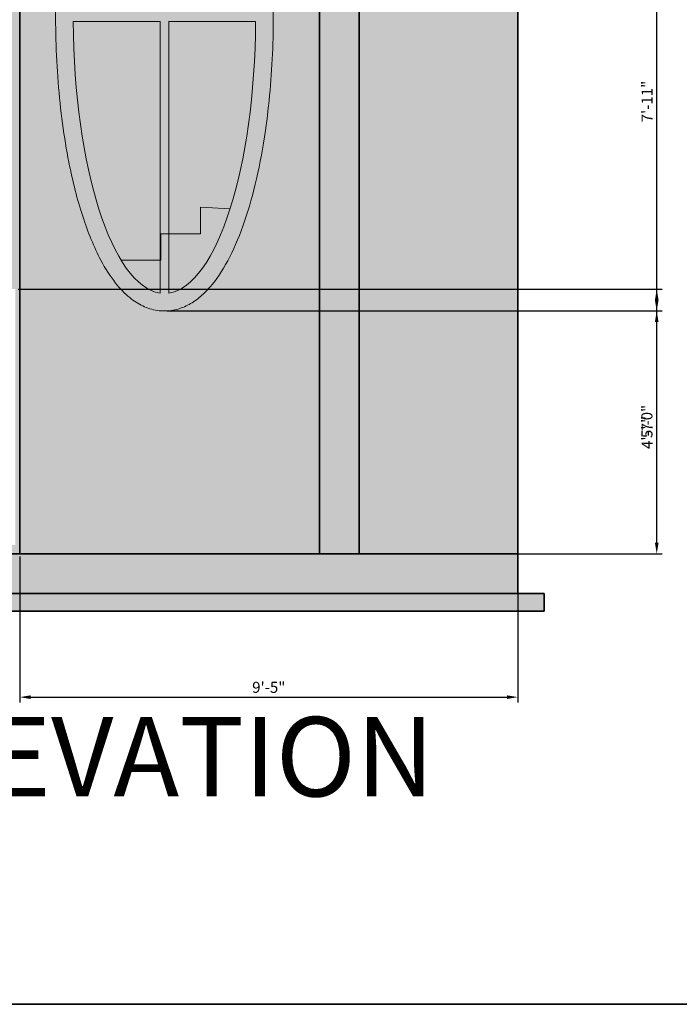
# Model space of a CAD drawing. Units: inches. Extents: x 2150 to 10686, y 1035 to 5077.
# Tile 6 of 12: x 6368 to 6517, y 4201 to 4425. Entities that reach past the tile are written whole.
import ezdxf

# ---------------------------------------------------------------- set-up
doc = ezdxf.new("R2010")
doc.units = ezdxf.units.IN
for name, color, linetype, lineweight in [('A-ANNO-DIMS', 2, 'Continuous', 18), ('A-ANNO-TITL', 3, 'Continuous', 35), ('A-ANNO-TTLB', 7, 'Continuous', 35), ('A-ELEV', 7, 'Continuous', 35), ('A-ELEV-BASE-PATT', 251, 'Continuous', 13), ('A-ELEV-GLAZ', 7, 'Continuous', 18), ('A-ELEV-METL-PATT', 252, 'Continuous', 13), ('A-ELEV-STRS', 7, 'Continuous', 18)]:
    doc.layers.add(name, color=color, linetype=linetype, lineweight=lineweight)
for name, color, linetype, lineweight, true_color in [('A-ELEV-CONC-PATT', 253, 'Continuous', 13, 0xb2a88f), ('A-ELEV-GLAZ-PATT', 141, 'Continuous', 13, 0xadddf7), ('A-ELEV-PATT', 253, 'Continuous', 13, 0xa5adc8), ('A-ELEV-TRIM-PATT', 85, 'Continuous', 13, 0x58ba48)]:
    doc.layers.add(name, color=color, linetype=linetype, lineweight=lineweight, true_color=true_color)
doc.styles.get("Standard").update_dxf_attribs({"font": 'arial.ttf'})
doc.dimstyles.new('ISO-25', dxfattribs={"dimtxt": 2.5, "dimasz": 2.5, "dimexe": 1.25, "dimexo": 0.625, "dimtad": 1, "dimdec": 0, "dimlunit": 3, "dimtxsty": 'Standard', "dimcen": 2.5, "dimadec": 0, "dimazin": 0, "dimtfac": 1, "dimtdec": 0, "dimtmove": 0, "dimatfit": 3, "dimfxl": 1, "dimarcsym": 0})

# ---------------------------------------------------------------- blocks, each defined once
blk = doc.blocks.new('*D130')
at = {"layer": 'A-ANNO-DIMS', "color": 0, "lineweight": -2, "transparency": 16777216}
for p, q in [((6401.069858000004, 4358.524472000001), (6513.357663000007, 4358.524472000001)), ((6512.107663000008, 4305.984460000001), (6512.107663000008, 4356.024472000002)), ((6481.232663000003, 4303.484460000001), (6513.357663000007, 4303.484460000001))]:
    blk.add_line(p, q, dxfattribs=at)
at = {"layer": 'A-ANNO-DIMS', "color": 0, "transparency": 16777216}
for points in [[(6511.69099633334, 4356.024472000002), (6512.524329666674, 4356.024472000002), (6512.107663000008, 4358.524472000001)], [(6511.69099633334, 4305.984460000001), (6512.524329666674, 4305.984460000001), (6512.107663000008, 4303.484460000001)]]:
    blk.add_solid(points, dxfattribs=at)
at = {"layer": 'Defpoints', "color": 0, "transparency": 16777216}
for p in [(6400.444858000003, 4358.524472000001), (6512.107663000008, 4358.524472000001), (6480.607663000004, 4303.484460000001)]:
    blk.add_point(p, dxfattribs=at)
at = {"layer": 'A-ANNO-DIMS', "color": 0, "transparency": 16777216, "insert": (6510.232663000007, 4331.004465999998), "char_height": 2.5, "attachment_point": 5, "rotation": 90}
blk.add_mtext('4\'-7"', dxfattribs=at)
blk = doc.blocks.new('*D131')
at = {"layer": 'A-ANNO-DIMS', "color": 0, "lineweight": -2, "transparency": 16777216}
for p, q in [((6493.232663000004, 4453.484460000001), (6513.357663000007, 4453.484460000001)), ((6512.107663000008, 4361.024472000002), (6512.107663000008, 4450.984460000001)), ((6401.069858000004, 4358.524472000001), (6513.357663000007, 4358.524472000001))]:
    blk.add_line(p, q, dxfattribs=at)
at = {"layer": 'A-ANNO-DIMS', "color": 0, "transparency": 16777216}
for points in [[(6511.69099633334, 4450.984460000001), (6512.524329666674, 4450.984460000001), (6512.107663000008, 4453.484460000001)], [(6511.69099633334, 4361.024472000002), (6512.524329666674, 4361.024472000002), (6512.107663000008, 4358.524472000001)]]:
    blk.add_solid(points, dxfattribs=at)
at = {"layer": 'Defpoints', "color": 0, "transparency": 16777216}
for p in [(6492.607663000004, 4453.484460000001), (6512.107663000008, 4453.484460000001), (6400.444858000003, 4358.524472000001)]:
    blk.add_point(p, dxfattribs=at)
at = {"layer": 'A-ANNO-DIMS', "color": 0, "transparency": 16777216, "insert": (6510.227547038205, 4406.004465999998), "char_height": 2.5, "attachment_point": 5, "rotation": 90}
blk.add_mtext('7\'-11"', dxfattribs=at)
blk = doc.blocks.new('*D135')
at = {"layer": 'A-ANNO-DIMS', "color": 0, "lineweight": -2, "transparency": 16777216}
for p, q in [((6367.607663, 4302.859459999999), (6367.607663, 4269.73446)), ((6480.607662999999, 4302.859459999999), (6480.607662999999, 4269.73446)), ((6370.107662999999, 4270.98446), (6478.107663, 4270.98446))]:
    blk.add_line(p, q, dxfattribs=at)
at = {"layer": 'A-ANNO-DIMS', "color": 0, "transparency": 16777216}
for points in [[(6370.107662999999, 4271.401126666666), (6370.107662999999, 4270.567793333333), (6367.607663, 4270.98446)], [(6478.107663, 4271.401126666666), (6478.107663, 4270.567793333333), (6480.607662999999, 4270.98446)]]:
    blk.add_solid(points, dxfattribs=at)
at = {"layer": 'Defpoints', "color": 0, "transparency": 16777216}
for p in [(6367.607663, 4303.484459999999), (6480.607662999999, 4303.484459999999), (6480.607662999999, 4270.98446)]:
    blk.add_point(p, dxfattribs=at)
at = {"layer": 'A-ANNO-DIMS', "color": 0, "transparency": 16777216, "insert": (6424.107663, 4272.885892469304), "char_height": 2.5, "attachment_point": 5}
blk.add_mtext('9\'-5"', dxfattribs=at)
blk = doc.blocks.new('*D137')
at = {"layer": 'A-ANNO-DIMS', "color": 0, "lineweight": -2, "transparency": 16777216}
for p, q in [((6367.232663000003, 4363.484460000001), (6513.357663000007, 4363.484460000001)), ((6512.107663000008, 4305.984460000001), (6512.107663000008, 4360.984460000001)), ((6368.232663000004, 4303.484460000001), (6513.357663000007, 4303.484460000001))]:
    blk.add_line(p, q, dxfattribs=at)
at = {"layer": 'A-ANNO-DIMS', "color": 0, "transparency": 16777216}
for points in [[(6511.69099633334, 4360.984460000001), (6512.524329666674, 4360.984460000001), (6512.107663000008, 4363.484460000001)], [(6511.69099633334, 4305.984460000001), (6512.524329666674, 4305.984460000001), (6512.107663000008, 4303.484460000001)]]:
    blk.add_solid(points, dxfattribs=at)
at = {"layer": 'Defpoints', "color": 0, "transparency": 16777216}
for p in [(6366.607663000003, 4363.484460000001), (6512.107663000008, 4363.484460000001), (6367.607663000003, 4303.484460000001)]:
    blk.add_point(p, dxfattribs=at)
at = {"layer": 'A-ANNO-DIMS', "color": 0, "transparency": 16777216, "insert": (6510.206230530702, 4333.484459999999), "char_height": 2.5, "attachment_point": 5, "rotation": 90}
blk.add_mtext('5\'-0"', dxfattribs=at)

msp = doc.modelspace()

# ---------------------------------------------------------------- hatches: boundary and pattern name
at = {"layer": 'A-ELEV-BASE-PATT'}
h = msp.add_hatch(color=256, dxfattribs=at)
h.dxf.hatch_style = 1
h.paths.add_polyline_path([(6480.633239304355, 4303.484460131323), (6240.6076634378, 4303.484460131323), (6240.6076634378, 4294.484460131323), (6480.633239304355, 4294.484460131323)])
h = msp.add_hatch(color=256, dxfattribs=at)
h.dxf.hatch_style = 1
h.paths.add_polyline_path([(6486.607663437801, 4294.484460131323), (6234.607663437801, 4294.484460131323), (6234.607663437801, 4290.484460131323), (6486.6076634378, 4290.484460131323)])
at = {"layer": 'A-ELEV-CONC-PATT'}
h = msp.add_hatch(dxfattribs=at)
h.set_pattern_fill('AR-CONC', color=256, scale=0.02)
h.set_pattern_definition([(50, (0, 0), (3.64369337992008, -0.3187817107780617), [0.381, -4.191]), (355, (0, 0), (-0.7048684284993869, 3.821136904780702), [0.3048, -3.3528116834]), (100.4514447, (0.30364014, -0.02656507), (2.938824941807065, 3.502355038243901), [0.323800176, -3.561804891999999]), (46.18420000000001, (0, 1.016), (5.421580817842598, -0.8408465586545428), [0.5714999999999999, -6.286499999999999]), (96.63555760999996, (0.4517980000000001, 0.94593), (4.74808268103006, 4.94852249195443), [0.4857004628000001, -5.342712163199999]), (351.18415117, (0, 1.016), (4.74808268129954, 4.948522491710653), [0.4571993414000001, -5.029194638399999]), (21, (0.508, 0.762), (3.032287825382649, -2.045303963741752), [0.381, -4.191]), (326, (0.508, 0.762), (1.236040566952941, 3.683759322446385), [0.3048, -3.352799999999999]), (71.45144499999999, (0.760690652, 0.5915580020000001), (4.268328385574323, 1.638455377718104), [0.323800176, -3.561798751999999]), (37.5, (0, 0), (0.0617720650118363, 1.691100777463062), [0, -3.312159999999999, 0, -3.4036, 0, -3.3655]), (7.499999999999999, (0, 0), (1.336393250206114, 2.00361149636239), [0, -1.940559999999999, 0, -3.235959999999999, 0, -1.2827]), (327.5, (-1.132839999999999, 0), (2.711811903337427, -0.1145748798534689), [0, -1.27, 0, -3.9624, 0, -5.257799999999999]), (317.5, (-1.64084, 0), (2.962583627720361, 0.5085298206666607), [0, -1.650999999999999, 0, -2.63144, 0, -3.7338])])
h.paths.add_polyline_path([(6444.633239304355, 4525.484460131322), (6367.6076634378, 4525.484460131324), (6367.6076634378, 4516.484460131324), (6435.633239304355, 4516.484460131323), (6435.633239304355, 4303.484460131323), (6444.633239304355, 4303.484460131323)])
h.paths.add_polyline_path([(6367.6076634378, 4453.484460131323), (6228.6076634378, 4453.484460131323), (6228.6076634378, 4447.484460131323), (6367.6076634378, 4447.484460131323)])
h.paths.add_polyline_path([(6492.607663437801, 4453.484460131323), (6480.633239304353, 4453.484460131322), (6480.633239304353, 4447.484460131323), (6492.607663437801, 4447.484460131323)])
h.paths.add_polyline_path([(6492.607663437801, 4554.484460131323), (6337.6076634378, 4554.484460131323), (6337.607663437799, 4549.484460131323), (6492.607663437799, 4549.484460131323)])
at = {"layer": 'A-ELEV-GLAZ-PATT'}
h = msp.add_hatch(color=256, dxfattribs=at)
h.dxf.hatch_style = 1
h.paths.add_polyline_path([(6279.607663437801, 4384.484460131323), (6267.607663437801, 4384.484460131323), (6267.6076634378, 4372.484460131324), (6279.607663437801, 4372.484460131324)])
h.paths.add_polyline_path([(6291.607663437801, 4384.484460131323), (6279.607663437801, 4384.484460131323), (6279.607663437801, 4372.484460131324), (6291.607663437801, 4372.484460131324)])
edge = h.paths.add_edge_path()
edge.add_ellipse((6400.444858416264, 4425.167712730096), major_axis=(0, -62.64324057997146), ratio=0.3301887017017349, start_angle=180.9156291084783, end_angle=267.2317619230999)
edge.add_line((6379.76340377621, 4426.167712730096), (6399.444858416265, 4426.167712730096))
edge.add_line((6399.444858416265, 4426.167712730096), (6399.444858416265, 4487.737700317675))
edge = h.paths.add_edge_path()
edge.add_ellipse((6400.444858416264, 4425.167712730096), major_axis=(0, -62.64324057997146), ratio=0.3301887017017349, start_angle=452.7682380769, end_angle=539.0843708915216)
edge.add_line((6401.444858416265, 4487.737700317675), (6401.444858416265, 4426.167712730096))
edge.add_line((6401.444858416265, 4426.167712730096), (6421.126313056319, 4426.167712730096))
edge = h.paths.add_edge_path()
edge.add_ellipse((6400.444858416264, 4425.167712730096), major_axis=(0, -62.64324057997146), ratio=0.3301887017017349, start_angle=378.88994340641, end_angle=447.2317619231)
edge.add_line((6421.126313056319, 4424.167712730096), (6401.444858416265, 4424.167712730096))
edge.add_line((6401.444858416265, 4424.167712730096), (6401.444858416265, 4376.02078865707))
edge.add_line((6401.444858416265, 4376.02078865707), (6408.633239304354, 4376.02078865707))
edge.add_line((6408.633239304354, 4376.02078865707), (6408.633239304354, 4382.020788657071))
edge.add_line((6408.633239304354, 4382.020788657071), (6415.329204846509, 4381.669182122283))
edge = h.paths.add_edge_path()
edge.add_line((6399.444858416265, 4424.167712730096), (6379.76340377621, 4424.167712730096))
edge.add_ellipse((6400.444858416264, 4425.167712730096), major_axis=(0, -62.64324057997146), ratio=0.3301887017017349, start_angle=272.7682380768999, end_angle=349.9116256040723)
edge.add_line((6390.633239304354, 4370.020788657071), (6399.444858416265, 4370.020788657071))
edge.add_line((6399.444858416265, 4370.020788657071), (6399.444858416265, 4424.167712730096))
edge = h.paths.add_edge_path()
edge.add_line((6399.444858416265, 4370.020788657071), (6390.633239304354, 4370.020788657071))
edge.add_ellipse((6400.444858416264, 4425.167712730096), major_axis=(0, -62.64324057997146), ratio=0.3301887017017349, start_angle=349.9116256040723, end_angle=359.0843708915216)
edge.add_line((6399.444858416265, 4362.597725142516), (6399.444858416265, 4370.020788657071))
edge = h.paths.add_edge_path()
edge.add_ellipse((6400.444858416264, 4425.167712730096), major_axis=(0, -62.64324057997146), ratio=0.3301887017017349, start_angle=360.9156291084783, end_angle=378.88994340641)
edge.add_line((6415.329204846509, 4381.669182122283), (6408.633239304354, 4382.020788657071))
edge.add_line((6408.633239304354, 4382.020788657071), (6408.633239304354, 4376.02078865707))
edge.add_line((6408.633239304354, 4376.02078865707), (6401.444858416265, 4376.02078865707))
edge.add_line((6401.444858416265, 4376.02078865707), (6401.444858416265, 4362.597725142516))
at = {"layer": 'A-ELEV-METL-PATT'}
h = msp.add_hatch(color=256, dxfattribs=at)
h.dxf.hatch_style = 1
edge = h.paths.add_edge_path()
edge.add_spline(control_points=[(6400.444858416264, 4358.524472150125), (6401.486440814489, 4358.524472150125), (6402.526505044808, 4358.677401357236), (6404.522486905328, 4359.255063234454), (6405.478003331038, 4359.677509034017), (6407.281736042183, 4360.731176144923), (6408.131339490663, 4361.361806443027), (6409.740207013673, 4362.793659380537), (6410.500149994661, 4363.595296803934), (6412.700838569434, 4366.265752912591), (6414.03394570237, 4368.379499630626), (6416.487744706213, 4373.197243253772), (6417.606172835956, 4375.903063890813), (6419.631029857393, 4381.840607040826), (6420.536486327513, 4385.072192199597), (6422.117938633519, 4391.962202533656), (6422.793588111736, 4395.620342382234), (6424.200323950252, 4405.332886237875), (6424.756775730746, 4411.600724829638), (6425.233072301224, 4424.345165291339), (6425.152698848673, 4430.819672112305), (6424.360861114452, 4443.427756971612), (6423.649784349251, 4449.559211921115), (6421.832101343849, 4459.914160022554), (6420.824100186611, 4464.280479948769), (6418.459699862937, 4472.224057176997), (6417.105531965493, 4475.800577784561), (6414.530984821721, 4481.046021704659), (6413.400413444257, 4482.963765924061), (6411.159609652, 4486.022314366695), (6410.081239671351, 4487.242292157316), (6407.981904490796, 4489.103336574784), (6406.994481886034, 4489.812440503778), (6404.88004816331, 4490.945334575583), (6403.750412373089, 4491.367263683768), (6401.591707320996, 4491.795744529485), (6400.578062848126, 4491.856564882596), (6398.574329452856, 4491.695615966483), (6397.586567833659, 4491.47475953499), (6395.700279883302, 4490.794741309719), (6394.801423289315, 4490.337316033343), (6393.101630982474, 4489.237707960262), (6392.299575991901, 4488.59571921333), (6390.776032761522, 4487.156246990203), (6390.054097434259, 4486.358390989495), (6387.868726596746, 4483.603993381065), (6386.519519142056, 4481.381571183187), (6384.042618140686, 4476.318979222956), (6382.917389359787, 4473.477169667343), (6380.892123096994, 4467.249882245213), (6379.993066323842, 4463.864616669574), (6378.439918554827, 4456.661812920038), (6377.786169577303, 4452.844597947903), (6376.462930365054, 4442.788115239438), (6375.974391004774, 4436.347147441612), (6375.659764204387, 4423.32378833974), (6375.833828926627, 4416.743682061819), (6376.8313878542, 4404.020783955098), (6377.654325200822, 4397.880344812312), (6379.642069279475, 4387.821914067098), (6380.689035460468, 4383.713325470128), (6383.106877716371, 4376.272307259607), (6384.47532253611, 4372.940336073535), (6387.048331366607, 4368.105027158752), (6388.164220640812, 4366.356485480582), (6390.369702204264, 4363.581332383819), (6391.427944586487, 4362.479757644216), (6393.496381316636, 4360.802633777571), (6394.475915167926, 4360.166036636088), (6396.563807655099, 4359.173441496676), (6397.674090126379, 4358.819701830231), (6399.355629057865, 4358.565786838256), (6399.900211293723, 4358.524472150125), (6400.444858416264, 4358.524472150125)], knot_values=[0, 0, 0, 0, 0.0952714022776172, 0.0952714022776172, 0.1905428045552344, 0.1905428045552344, 0.2858142068328516, 0.2858142068328516, 0.3810856091104688, 0.3810856091104688, 0.575169634462188, 0.575169634462188, 0.7692536598139071, 0.7692536598139071, 0.9633376851656262, 0.9633376851656262, 1.157421710517345, 1.157421710517345, 1.458089536658081, 1.458089536658081, 1.758757362798818, 1.758757362798818, 2.059425188939554, 2.059425188939554, 2.304413142887573, 2.304413142887573, 2.549401096835591, 2.549401096835591, 2.718168677128249, 2.718168677128249, 2.856837524264077, 2.856837524264077, 2.966492349551455, 2.966492349551455, 3.076147174838833, 3.076147174838833, 3.168108685177037, 3.168108685177037, 3.260070195515242, 3.260070195515242, 3.352031705853447, 3.352031705853447, 3.443993216191651, 3.443993216191651, 3.535954726529856, 3.535954726529856, 3.735259798893268, 3.735259798893268, 3.93456487125668, 3.93456487125668, 4.133869943620092, 4.133869943620092, 4.333175015983504, 4.333175015983504, 4.639352924429541, 4.639352924429541, 4.945530832875578, 4.945530832875578, 5.251708741321616, 5.251708741321616, 5.489766878495931, 5.489766878495931, 5.727825015670246, 5.727825015670246, 5.88940932659502, 5.88940932659502, 6.02159730311115, 6.02159730311115, 6.127482428421133, 6.127482428421133, 6.233367553731117, 6.233367553731117, 6.283185307179586, 6.283185307179586, 6.283185307179586, 6.283185307179586], degree=3, periodic=0)
edge = h.paths.add_edge_path(flags=16)
edge.add_line((6399.444858416265, 4487.737700317675), (6399.444858416265, 4426.167712730096))
edge.add_line((6399.444858416265, 4426.167712730096), (6379.76340377621, 4426.167712730096))
edge.add_ellipse((6400.444858416264, 4425.167712730096), major_axis=(0, -62.64324057997146), ratio=0.3301887017017349, start_angle=180.9156291084783, end_angle=267.2317619230999, ccw=False)
edge = h.paths.add_edge_path(flags=16)
edge.add_ellipse((6400.444858416264, 4425.167712730096), major_axis=(0, -62.64324057997146), ratio=0.3301887017017349, start_angle=452.7682380769001, end_angle=539.0843708915218, ccw=False)
edge.add_line((6421.126313056319, 4426.167712730096), (6401.444858416265, 4426.167712730096))
edge.add_line((6401.444858416265, 4426.167712730096), (6401.444858416265, 4487.737700317675))
edge = h.paths.add_edge_path(flags=16)
edge.add_line((6399.444858416265, 4424.167712730097), (6399.444858416265, 4370.020788657071))
edge.add_line((6399.444858416265, 4370.020788657071), (6399.633239304353, 4370.020788657071))
edge.add_line((6399.633239304353, 4370.020788657071), (6399.633239304353, 4376.02078865707))
edge.add_line((6399.633239304353, 4376.02078865707), (6401.444858416265, 4376.02078865707))
edge.add_line((6401.444858416265, 4376.02078865707), (6401.444858416265, 4424.167712730096))
edge.add_line((6401.444858416265, 4424.167712730096), (6421.126313056319, 4424.167712730096))
edge.add_ellipse((6400.444858416264, 4425.167712730096), major_axis=(0, -62.64324057997146), ratio=0.3301887017017349, start_angle=378.88994340641005, end_angle=447.23176192310007, ccw=False)
edge.add_ellipse((6400.444858416264, 4425.167712730096), major_axis=(0, -62.64324057997146), ratio=0.3301887017017349, start_angle=360.9156291084783, end_angle=378.88994340641005, ccw=False)
edge.add_line((6401.444858416265, 4362.597725142516), (6401.444858416265, 4376.02078865707))
edge.add_line((6401.444858416265, 4376.02078865707), (6399.633239304353, 4376.02078865707))
edge.add_line((6399.633239304353, 4376.02078865707), (6399.633239304353, 4370.020788657071))
edge.add_line((6399.633239304353, 4370.020788657071), (6399.444858416265, 4370.020788657071))
edge.add_line((6399.444858416265, 4370.020788657071), (6399.444858416265, 4362.597725142516))
edge.add_ellipse((6400.444858416264, 4425.167712730096), major_axis=(0, -62.64324057997146), ratio=0.3301887017017349, start_angle=349.9116256040723, end_angle=359.0843708915217, ccw=False)
edge.add_ellipse((6400.444858416264, 4425.167712730096), major_axis=(0, -62.64324057997146), ratio=0.3301887017017349, start_angle=272.76823807689993, end_angle=349.9116256040723, ccw=False)
edge.add_line((6379.76340377621, 4424.167712730096), (6399.444858416265, 4424.167712730097))
h.paths.add_polyline_path([(6294.607663437801, 4387.484460131323), (6264.6076634378, 4387.484460131323), (6264.6076634378, 4369.484460131324), (6294.607663437801, 4369.484460131324)])
h.paths.add_polyline_path([(6267.607663437801, 4384.484460131323), (6291.607663437801, 4384.484460131323), (6291.607663437801, 4372.484460131324), (6267.6076634378, 4372.484460131324)], flags=16)
at = {"layer": 'A-ELEV-PATT'}
h = msp.add_hatch(color=256, dxfattribs=at)
h.dxf.hatch_style = 1
h.paths.add_polyline_path([(6435.633239304355, 4516.484460131323), (6367.6076634378, 4516.484460131324), (6367.6076634378, 4303.484460131323), (6435.633239304355, 4303.484460131323)])
edge = h.paths.add_edge_path(flags=16)
edge.add_spline(control_points=[(6400.444858416264, 4358.524472150125), (6401.486440814489, 4358.524472150125), (6402.526505044808, 4358.677401357236), (6404.522486905328, 4359.255063234454), (6405.478003331038, 4359.677509034017), (6407.281736042183, 4360.731176144923), (6408.131339490663, 4361.361806443027), (6409.740207013673, 4362.793659380537), (6410.500149994661, 4363.595296803934), (6412.700838569434, 4366.265752912591), (6414.03394570237, 4368.379499630626), (6416.487744706213, 4373.197243253772), (6417.606172835956, 4375.903063890813), (6419.631029857393, 4381.840607040826), (6420.536486327513, 4385.072192199597), (6422.117938633519, 4391.962202533656), (6422.793588111736, 4395.620342382234), (6424.200323950252, 4405.332886237875), (6424.756775730746, 4411.600724829638), (6425.233072301224, 4424.345165291339), (6425.152698848673, 4430.819672112305), (6424.360861114452, 4443.427756971612), (6423.649784349251, 4449.559211921115), (6421.832101343849, 4459.914160022554), (6420.824100186611, 4464.280479948769), (6418.459699862937, 4472.224057176997), (6417.105531965493, 4475.800577784561), (6414.530984821721, 4481.046021704659), (6413.400413444257, 4482.963765924061), (6411.159609652, 4486.022314366695), (6410.081239671351, 4487.242292157316), (6407.981904490796, 4489.103336574784), (6406.994481886034, 4489.812440503778), (6404.88004816331, 4490.945334575583), (6403.750412373089, 4491.367263683768), (6401.591707320996, 4491.795744529485), (6400.578062848126, 4491.856564882596), (6398.574329452856, 4491.695615966483), (6397.586567833659, 4491.47475953499), (6395.700279883302, 4490.794741309719), (6394.801423289315, 4490.337316033343), (6393.101630982474, 4489.237707960262), (6392.299575991901, 4488.59571921333), (6390.776032761522, 4487.156246990203), (6390.054097434259, 4486.358390989495), (6387.868726596746, 4483.603993381065), (6386.519519142056, 4481.381571183187), (6384.042618140686, 4476.318979222956), (6382.917389359787, 4473.477169667343), (6380.892123096994, 4467.249882245213), (6379.993066323842, 4463.864616669574), (6378.439918554827, 4456.661812920038), (6377.786169577303, 4452.844597947903), (6376.462930365054, 4442.788115239438), (6375.974391004774, 4436.347147441612), (6375.659764204387, 4423.32378833974), (6375.833828926627, 4416.743682061819), (6376.8313878542, 4404.020783955098), (6377.654325200822, 4397.880344812312), (6379.642069279475, 4387.821914067098), (6380.689035460468, 4383.713325470128), (6383.106877716371, 4376.272307259607), (6384.47532253611, 4372.940336073535), (6387.048331366607, 4368.105027158752), (6388.164220640812, 4366.356485480582), (6390.369702204264, 4363.581332383819), (6391.427944586487, 4362.479757644216), (6393.496381316636, 4360.802633777571), (6394.475915167926, 4360.166036636088), (6396.563807655099, 4359.173441496676), (6397.674090126379, 4358.819701830231), (6399.355629057865, 4358.565786838256), (6399.900211293723, 4358.524472150125), (6400.444858416264, 4358.524472150125)], knot_values=[0, 0, 0, 0, 0.0952714022776172, 0.0952714022776172, 0.1905428045552344, 0.1905428045552344, 0.2858142068328516, 0.2858142068328516, 0.3810856091104688, 0.3810856091104688, 0.575169634462188, 0.575169634462188, 0.7692536598139071, 0.7692536598139071, 0.9633376851656262, 0.9633376851656262, 1.157421710517345, 1.157421710517345, 1.458089536658081, 1.458089536658081, 1.758757362798818, 1.758757362798818, 2.059425188939554, 2.059425188939554, 2.304413142887573, 2.304413142887573, 2.549401096835591, 2.549401096835591, 2.718168677128249, 2.718168677128249, 2.856837524264077, 2.856837524264077, 2.966492349551455, 2.966492349551455, 3.076147174838833, 3.076147174838833, 3.168108685177037, 3.168108685177037, 3.260070195515242, 3.260070195515242, 3.352031705853447, 3.352031705853447, 3.443993216191651, 3.443993216191651, 3.535954726529856, 3.535954726529856, 3.735259798893268, 3.735259798893268, 3.93456487125668, 3.93456487125668, 4.133869943620092, 4.133869943620092, 4.333175015983504, 4.333175015983504, 4.639352924429541, 4.639352924429541, 4.945530832875578, 4.945530832875578, 5.251708741321616, 5.251708741321616, 5.489766878495931, 5.489766878495931, 5.727825015670246, 5.727825015670246, 5.88940932659502, 5.88940932659502, 6.02159730311115, 6.02159730311115, 6.127482428421133, 6.127482428421133, 6.233367553731117, 6.233367553731117, 6.283185307179586, 6.283185307179586, 6.283185307179586, 6.283185307179586], degree=3, periodic=0)
edge = h.paths.add_edge_path(flags=0)
edge.add_ellipse((6400.444858416264, 4425.167712730096), major_axis=(0, -62.64324057997146), ratio=0.3301887017017349, start_angle=452.7682380769001, end_angle=539.0843708915218, ccw=False)
edge.add_line((6421.126313056319, 4426.167712730096), (6401.444858416265, 4426.167712730096))
edge.add_line((6401.444858416265, 4426.167712730096), (6401.444858416265, 4487.737700317675))
edge = h.paths.add_edge_path(flags=0)
edge.add_line((6399.444858416265, 4487.737700317675), (6399.444858416265, 4426.167712730096))
edge.add_line((6399.444858416265, 4426.167712730096), (6379.76340377621, 4426.167712730096))
edge.add_ellipse((6400.444858416264, 4425.167712730096), major_axis=(0, -62.64324057997146), ratio=0.3301887017017349, start_angle=180.9156291084783, end_angle=267.2317619230999, ccw=False)
edge = h.paths.add_edge_path(flags=0)
edge.add_ellipse((6400.444858416264, 4425.167712730096), major_axis=(0, -62.64324057997146), ratio=0.3301887017017349, start_angle=378.88994340641005, end_angle=447.23176192310007, ccw=False)
edge.add_ellipse((6400.444858416264, 4425.167712730096), major_axis=(0, -62.64324057997146), ratio=0.3301887017017349, start_angle=360.9156291084783, end_angle=378.88994340641005, ccw=False)
edge.add_line((6401.444858416265, 4362.597725142516), (6401.444858416265, 4376.02078865707))
edge.add_line((6401.444858416265, 4376.02078865707), (6399.633239304353, 4376.02078865707))
edge.add_line((6399.633239304353, 4376.02078865707), (6399.633239304353, 4370.020788657071))
edge.add_line((6399.633239304353, 4370.020788657071), (6399.444858416265, 4362.597725142516))
edge.add_ellipse((6400.444858416264, 4425.167712730096), major_axis=(0, -62.64324057997146), ratio=0.3301887017017349, start_angle=349.9116256040723, end_angle=359.0843708915217, ccw=False)
edge.add_ellipse((6400.444858416264, 4425.167712730096), major_axis=(0, -62.64324057997146), ratio=0.3301887017017349, start_angle=272.76823807689993, end_angle=349.9116256040723, ccw=False)
edge.add_line((6379.76340377621, 4424.167712730096), (6399.444858416265, 4424.167712730096))
edge.add_line((6399.444858416265, 4424.167712730096), (6399.444858416265, 4376.02078865707))
edge.add_line((6399.444858416265, 4376.02078865707), (6401.444858416265, 4376.02078865707))
edge.add_line((6401.444858416265, 4376.02078865707), (6401.444858416265, 4424.167712730096))
edge.add_line((6401.444858416265, 4424.167712730096), (6421.126313056319, 4424.167712730096))
h = msp.add_hatch(color=256, dxfattribs=at)
h.dxf.hatch_style = 1
h.paths.add_polyline_path([(6367.6076634378, 4447.484460131323), (6318.6076634378, 4447.484460131323), (6318.607663437799, 4303.484460131323), (6319.607663437792, 4303.484460131323), (6319.607663437802, 4387.484460131323), (6355.607663437799, 4387.484460131323), (6355.607663437799, 4363.484460131324), (6366.607663437799, 4363.484460131324), (6366.6076634378, 4305.484460131324), (6320.6076634378, 4305.484460131324), (6320.6076634378, 4303.484460131323), (6367.6076634378, 4303.484460131323)])
at = {"layer": 'A-ELEV-TRIM-PATT'}
h = msp.add_hatch(color=256, dxfattribs=at)
h.dxf.hatch_style = 1
h.paths.add_polyline_path([(6480.633239304353, 4549.484460131323), (6367.6076634378, 4549.484460131323), (6367.6076634378, 4525.484460131324), (6444.633239304355, 4525.484460131322), (6444.633239304355, 4303.484460131323), (6480.633239304355, 4303.484460131323)])

# ---------------------------------------------------------------- linework, layer by layer
at = {"layer": 'A-ANNO-TTLB'}
msp.add_lwpolyline([(6112.690859240117, 5076.611187983804), (7001.249989206184, 5076.611187983804), (7001.249989206184, 4201.352691599126), (6112.690859240117, 4201.352691599126)], close=True, dxfattribs=at)
at = {"layer": 'A-ELEV'}
for p, q in [((6367.6076634378, 4549.484460131323), (6367.6076634378, 4303.484460131323)), ((6480.633239304355, 4294.484460131323), (6480.633239304353, 4549.484460131323)), ((6444.633239304355, 4303.484460131323), (6444.633239304355, 4525.484460131323)), ((6435.633239304355, 4303.484460131323), (6435.633239304355, 4516.484460131322)), ((6240.6076634378, 4303.484460131323), (6480.6076634378, 4303.484460131323)), ((6234.607663437801, 4294.484460131323), (6486.6076634378, 4294.484460131323)), ((6486.607663437801, 4294.484460131323), (6486.6076634378, 4290.484460131323)), ((6234.607663437801, 4290.484460131323), (6486.6076634378, 4290.484460131323))]:
    msp.add_line(p, q, dxfattribs=at)
at = {"layer": 'A-ELEV-GLAZ'}
for p, q in [((6379.76340377621, 4424.167712730096), (6399.444858416265, 4424.167712730096)), ((6399.444858416265, 4424.167712730097), (6399.444858416265, 4362.597725142516)), ((6401.444858416265, 4424.167712730096), (6421.126313056319, 4424.167712730096)), ((6401.444858416265, 4424.167712730096), (6401.444858416265, 4362.597725142516))]:
    msp.add_line(p, q, dxfattribs=at)
for start_param, end_param in [(4.728353072717369, 6.23482011643244), (6.331550497926731, 7.838017541641803)]:
    msp.add_ellipse((6400.444858416264, 4425.167712730096), major_axis=(0, -62.64324057997146), ratio=0.3301887017017349, start_param=start_param, end_param=end_param, dxfattribs=at)
msp.add_open_spline([(6400.444858416264, 4358.524472150125), (6401.486440814489, 4358.524472150125), (6402.526505044808, 4358.677401357236), (6404.522486905328, 4359.255063234454), (6405.478003331038, 4359.677509034017), (6407.281736042183, 4360.731176144923), (6408.131339490663, 4361.361806443027), (6409.740207013673, 4362.793659380537), (6410.500149994661, 4363.595296803934), (6412.700838569434, 4366.265752912591), (6414.03394570237, 4368.379499630626), (6416.487744706213, 4373.197243253772), (6417.606172835956, 4375.903063890813), (6419.631029857393, 4381.840607040826), (6420.536486327513, 4385.072192199597), (6422.117938633519, 4391.962202533656), (6422.793588111736, 4395.620342382234), (6424.200323950252, 4405.332886237875), (6424.756775730746, 4411.600724829638), (6425.233072301224, 4424.345165291339), (6425.152698848673, 4430.819672112305), (6424.360861114452, 4443.427756971612), (6423.649784349251, 4449.559211921115), (6421.832101343849, 4459.914160022554), (6420.824100186611, 4464.280479948769), (6418.459699862937, 4472.224057176997), (6417.105531965493, 4475.800577784561), (6414.530984821721, 4481.046021704659), (6413.400413444257, 4482.963765924061), (6411.159609652, 4486.022314366695), (6410.081239671351, 4487.242292157316), (6407.981904490796, 4489.103336574784), (6406.994481886034, 4489.812440503778), (6404.88004816331, 4490.945334575583), (6403.750412373089, 4491.367263683768), (6401.591707320996, 4491.795744529485), (6400.578062848126, 4491.856564882596), (6398.574329452856, 4491.695615966483), (6397.586567833659, 4491.47475953499), (6395.700279883302, 4490.794741309719), (6394.801423289315, 4490.337316033343), (6393.101630982474, 4489.237707960262), (6392.299575991901, 4488.59571921333), (6390.776032761522, 4487.156246990203), (6390.054097434259, 4486.358390989495), (6387.868726596746, 4483.603993381065), (6386.519519142056, 4481.381571183187), (6384.042618140686, 4476.318979222956), (6382.917389359787, 4473.477169667343), (6380.892123096994, 4467.249882245213), (6379.993066323842, 4463.864616669574), (6378.439918554827, 4456.661812920038), (6377.786169577303, 4452.844597947903), (6376.462930365054, 4442.788115239438), (6375.974391004774, 4436.347147441612), (6375.659764204387, 4423.32378833974), (6375.833828926627, 4416.743682061819), (6376.8313878542, 4404.020783955098), (6377.654325200822, 4397.880344812312), (6379.642069279475, 4387.821914067098), (6380.689035460468, 4383.713325470128), (6383.106877716371, 4376.272307259607), (6384.47532253611, 4372.940336073535), (6387.048331366607, 4368.105027158752), (6388.164220640812, 4366.356485480582), (6390.369702204264, 4363.581332383819), (6391.427944586487, 4362.479757644216), (6393.496381316636, 4360.802633777571), (6394.475915167926, 4360.166036636088), (6396.563807655099, 4359.173441496676), (6397.674090126379, 4358.819701830231), (6399.355629057865, 4358.565786838256), (6399.900211293723, 4358.524472150125), (6400.444858416264, 4358.524472150125)], degree=3, knots=[0, 0, 0, 0, 0.0952714022776172, 0.0952714022776172, 0.1905428045552344, 0.1905428045552344, 0.2858142068328516, 0.2858142068328516, 0.3810856091104688, 0.3810856091104688, 0.575169634462188, 0.575169634462188, 0.7692536598139071, 0.7692536598139071, 0.9633376851656262, 0.9633376851656262, 1.157421710517345, 1.157421710517345, 1.458089536658081, 1.458089536658081, 1.758757362798818, 1.758757362798818, 2.059425188939554, 2.059425188939554, 2.304413142887573, 2.304413142887573, 2.549401096835591, 2.549401096835591, 2.718168677128249, 2.718168677128249, 2.856837524264077, 2.856837524264077, 2.966492349551455, 2.966492349551455, 3.076147174838833, 3.076147174838833, 3.168108685177037, 3.168108685177037, 3.260070195515242, 3.260070195515242, 3.352031705853447, 3.352031705853447, 3.443993216191651, 3.443993216191651, 3.535954726529856, 3.535954726529856, 3.735259798893268, 3.735259798893268, 3.93456487125668, 3.93456487125668, 4.133869943620092, 4.133869943620092, 4.333175015983504, 4.333175015983504, 4.639352924429541, 4.639352924429541, 4.945530832875578, 4.945530832875578, 5.251708741321616, 5.251708741321616, 5.489766878495931, 5.489766878495931, 5.727825015670246, 5.727825015670246, 5.88940932659502, 5.88940932659502, 6.02159730311115, 6.02159730311115, 6.127482428421133, 6.127482428421133, 6.233367553731117, 6.233367553731117, 6.283185307179586, 6.283185307179586, 6.283185307179586, 6.283185307179586], dxfattribs=at)
at = {"layer": 'A-ELEV-STRS'}
for p, q in [((6408.633239304354, 4376.02078865707), (6408.633239304354, 4382.020788657071)), ((6408.633239304354, 4382.020788657071), (6415.329204846509, 4381.669182122283)), ((6399.633239304353, 4370.020788657071), (6399.633239304353, 4376.02078865707)), ((6399.633239304353, 4376.02078865707), (6408.633239304354, 4376.02078865707)), ((6390.633239304354, 4370.020788657071), (6399.633239304353, 4370.020788657071))]:
    msp.add_line(p, q, dxfattribs=at)

# ---------------------------------------------------------------- texts
at = {"layer": 'A-ANNO-TITL', "insert": (6247.142359601145, 4266.476998592536), "char_height": 18, "attachment_point": 1}
msp.add_mtext_dynamic_manual_height_columns('FRONT ELEVATION', width=338.5750231852289, gutter_width=12.5, heights=[0], dxfattribs=at)

# ---------------------------------------------------------------- dimensions: what is measured, and where the dimension line sits
at = {"layer": 'A-ANNO-DIMS'}
for base, p1, p2, picture, middle in [((6512.107663000008, 4453.484460000001), (6400.444858, 4358.524472), (6492.607663, 4453.48446), '*D131', (6510.227547038205, 4406.004465999998)), ((6512.107663000008, 4363.484460000001), (6367.607663, 4303.484459999999), (6366.607662999999, 4363.48446), '*D137', (6510.206230530702, 4333.484459999999)), ((6512.107663000008, 4358.524472000001), (6480.607662999999, 4303.484459999999), (6400.444858, 4358.524472), '*D130', (6510.232663000007, 4331.004465999998))]:
    dim = msp.add_linear_dim(base=base, p1=p1, p2=p2, angle=90, dimstyle='ISO-25', override={"dimdec": 1, "dimlfac": 1, "dimrnd": 0, "dimzin": 1, "dimdsep": 46, "dimlunit": 4, "dimfrac": 2}, dxfattribs=at)
    dim.commit()
    dim.dimension.update_dxf_attribs({"geometry": picture, "text_midpoint": middle})
dim = msp.add_linear_dim(base=(6480.607662999999, 4270.98446), p1=(6367.607663, 4303.484459999999), p2=(6480.607662999999, 4303.484459999999), dimstyle='ISO-25', override={"dimdec": 1, "dimlfac": 1, "dimrnd": 0, "dimzin": 1, "dimdsep": 46, "dimlunit": 4, "dimfrac": 2}, dxfattribs=at)
dim.commit()
dim.dimension.update_dxf_attribs({"geometry": '*D135', "text_midpoint": (6424.107663, 4272.885892469304)})

doc.saveas('drawing.dxf')
